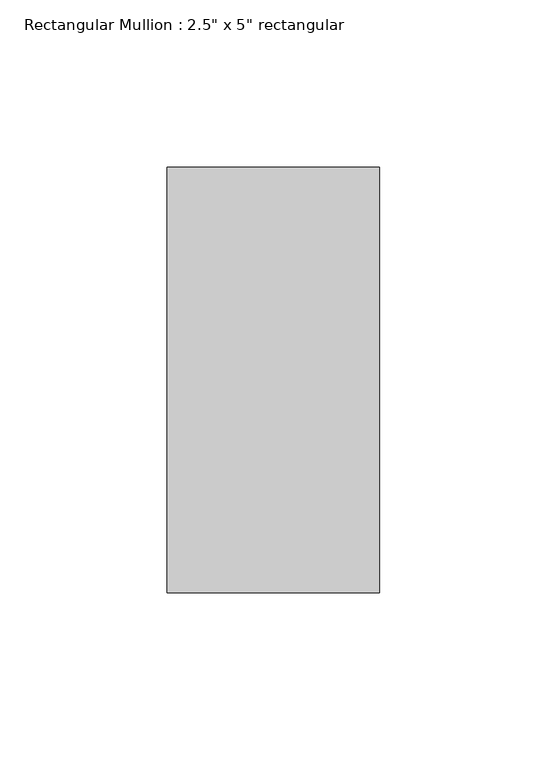
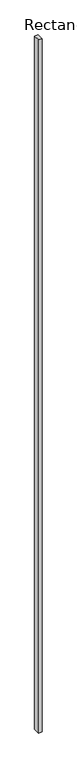
"""IFC4 building model written with IfcOpenShell, lengths in millimetres: member geometry."""

from ifc_helpers import new_model, si_unit, frame, origin, place, context, project, spatial, polyline, outline, extrude, source, transform, mapped, element, save


def member_b978f1c8(model_context):
    return source(origin(), model_context, "Body", "SweptSolid", [
        extrude(outline(polyline([(0.0, 63.5), (0.0, -63.5), (-63.5, -63.5), (-63.5, 63.5), (0.0, 63.5)])), frame((0.0, 0.0, -13703.3), z_axis=(0.0, 0.0, 1.0), x_axis=(1.0, 0.0, 0.0)), (0.0, 0.0, 1.0), 13703.3),
    ])


if __name__ == "__main__":
    model = new_model("IFC4")
    model_context = context("Model", 3, world=origin())
    ifc_project = project(units=[si_unit("LENGTHUNIT", "METRE", prefix="MILLI")], contexts=[model_context])
    site = spatial("IfcSite", under=ifc_project)
    building = spatial("IfcBuilding", under=site)
    placement = place(None, origin())
    member_shape = member_b978f1c8(model_context)
    element("IfcMember", 1, ObjectType="Rectangular Mullion : 2.5\" x 5\" rectangular", at=placement, inside=building, context=model_context, shape_type="MappedRepresentation", body=[
        mapped(member_shape, transform((0.0, 0.0, 0.0), x_axis=(1.0, 0.0, 0.0), y_axis=(0.0, 1.0, 0.0), z_axis=(0.0, 0.0, 1.0))),
    ])
    save(model, "model.ifc")

# Revit data of these elements
# Type "Rectangular Mullion : 2.5\" x 5\" rectangular"
#   built-in parameter 1007304 = 0.416667 (stored number, unit not read)
#   built-in parameter 1007301 = 0.104167 (stored number, unit not read)
#   built-in parameter 1007300 = 0.104167 (stored number, unit not read)
# Element 1 (IfcMember, "Rectangular Mullion : 2.5\" x 5\" rectangular")
#   Materials on its faces: "Aluminum"
# Materials
#   "Aluminum": class "Metal", colour RGB 247 247 247, transparency 0, Description = "Aluminum 6061", Cost = 0
